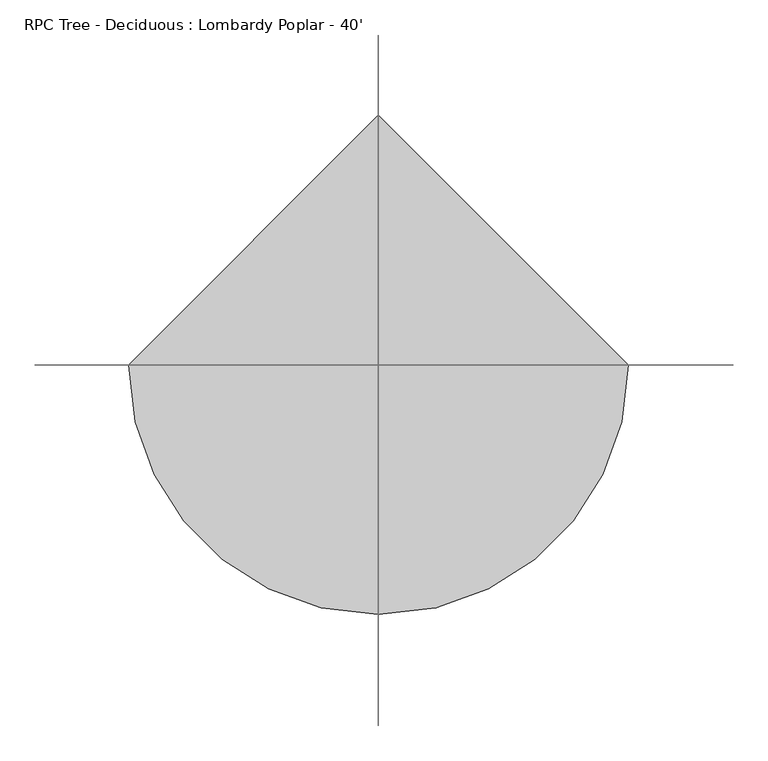
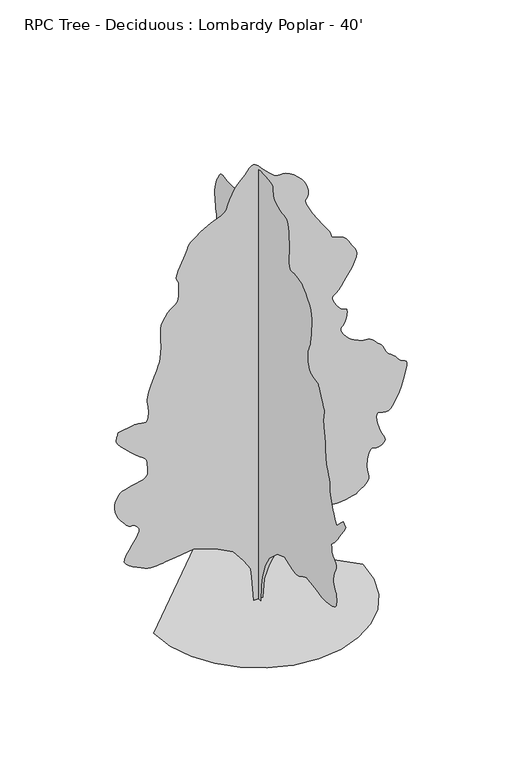
"""IFC4 building model written with IfcOpenShell, lengths in millimetres: geographic element geometry, RPC Tree - Deciduous : Lombardy Poplar - 40'."""

from ifc_helpers import new_model, si_unit, origin, place, context, project, spatial, triangles, source, transform, mapped, element, save


def rpc_tree_deciduous_lombardy_poplar_40_01077960(model_context):
    return source(origin(), model_context, "Body", "Tessellation", [
        triangles([(0.0009695, 113.8156909, 0.0), (0.0009695, -104.8345258, 0.0), (0.0009695, -123.055434, 437.3009239), (0.0009695, -177.7179314, 728.8340738), (0.0009695, -323.483707, 1129.6911467), (0.0009695, -505.6928613, 1439.4461494), (0.0009695, -870.1086628, 1767.420607), (0.0009695, -1216.3049732, 1894.9664555), (0.0009695, -1398.5142002, 1822.0838402), (0.0009695, -1476.390406, 1795.1523445), (0.0009695, -1552.9941605, 1770.6083485), (0.0009695, -1627.0451637, 1750.8472), (0.0009695, -1697.2735806, 1738.2588696), (0.0009695, -1762.3991112, 1735.2286766), (0.0009695, -1821.1516296, 1744.1542946), (0.0009695, -1872.2563591, 1767.420607), (0.0009695, -1919.1091679, 1797.0624023), (0.0009695, -1965.9644474, 1823.8364948), (0.0009695, -2012.8172562, 1848.2204716), (0.0009695, -2059.6700649, 1870.6891582), (0.0009695, -2106.5227283, 1891.7279903), (0.0009695, -2153.3780079, 1911.8067066), (0.0009695, -2200.2308167, 1931.4103065), (0.0009695, -2582.8711235, 1876.7470734), (0.0009695, -2649.2156204, 1861.2353748), (0.0009695, -2715.4080917, 1846.3611374), (0.0009695, -2781.27006, 1832.7619675), (0.0009695, -2846.6750793, 1821.0754715), (0.0009695, -2911.4196739, 1811.9366398), (0.0009695, -2975.3765259, 1805.987875), (0.0009695, -3038.3939003, 1803.8619873), (0.0009695, -3111.6472778, 1806.252103), (0.0009695, -3200.5217949, 1814.0625275), (0.0009695, -3296.0764275, 1828.2459641), (0.0009695, -3389.4213112, 1849.7596218), (0.0009695, -3471.5901329, 1879.5614365), (0.0009695, -3533.6930283, 1918.6062916), (0.0009695, -3566.7892639, 1967.8516869), (0.0009695, -3579.2353065, 2021.4507408), (0.0009695, -3585.9154221, 2073.1371208), (0.0009695, -3587.8205383, 2123.2333363), (0.0009695, -3585.9154221, 2172.0521587), (0.0009695, -3581.1401321, 2219.915807), (0.0009695, -3574.4347275, 2267.139378), (0.0009695, -3566.7892639, 2314.0455265), (0.0009695, -3532.0422569, 2353.5170998), (0.0009695, -3499.7078934, 2395.5361919), (0.0009695, -3472.1235306, 2442.6555542), (0.0009695, -3451.7273918, 2497.4231415), (0.0009695, -3440.907122, 2562.3988266), (0.0009695, -3441.9992065, 2640.0972816), (0.0009695, -3457.4677391, 2733.1372421), (0.0009695, -3484.5187042, 2825.1865654), (0.0009695, -3515.3799019, 2900.6752716), (0.0009695, -3544.9708282, 2963.0830902), (0.0009695, -3568.1862717, 3015.940329), (0.0009695, -3579.9210205, 3062.7525879), (0.0009695, -3575.0695724, 3106.9993057), (0.0009695, -3548.5775848, 3152.2110809), (0.0009695, -3509.7918709, 3193.1050964), (0.0009695, -3472.6063499, 3225.0836678), (0.0009695, -3438.6212151, 3252.6171616), (0.0009695, -3409.3857903, 3280.1253662), (0.0009695, -3386.5511375, 3312.1039375), (0.0009695, -3371.6668716, 3352.997953), (0.0009695, -3366.3581841, 3407.3030685), (0.0009695, -3362.7005585, 3460.5158089), (0.0009695, -3354.9027786, 3498.4634926), (0.0009695, -3347.7145546, 3525.8699593), (0.0009695, -3345.9620453, 3547.5360786), (0.0009695, -3354.4202499, 3568.2624298), (0.0009695, -3377.8388786, 3592.7987228), (0.0009695, -3421.0188011, 3625.9458275), (0.0009695, -3481.5215034, 3679.8698616), (0.0009695, -3552.5654228, 3760.5655174), (0.0009695, -3632.3465996, 3863.5624283), (0.0009695, -3719.1381042, 3984.4155167), (0.0009695, -3811.2130074, 4118.6541252), (0.0009695, -3906.7676399, 4261.8084686), (0.0009695, -4004.1003616, 4409.432888), (0.0009695, -3894.7788368, 4518.779702), (0.0009695, -3749.0086647, 4391.221209), (0.0009695, -3603.2382019, 4227.2390671), (0.0009695, -3579.7434151, 4258.785688), (0.0009695, -3555.9689941, 4292.2630051), (0.0009695, -3531.5088593, 4329.5499733), (0.0009695, -3506.1342453, 4372.5775795), (0.0009695, -3479.4643616, 4423.2506493), (0.0009695, -3451.1939941, 4483.4992973), (0.0009695, -3421.0188011, 4555.2033508), (0.0009695, -3390.0055779, 4628.5837555), (0.0009695, -3360.2623352, 4695.8683113), (0.0009695, -3333.0587631, 4762.2383881), (0.0009695, -3309.6910034, 4832.7233299), (0.0009695, -3291.4028755, 4912.4536377), (0.0009695, -3279.5158104, 5006.5351044), (0.0009695, -3275.248629, 5120.0473618), (0.0009695, -3267.0697678, 5234.8554703), (0.0009695, -3245.5050957, 5333.3820145), (0.0009695, -3215.0252701, 5421.7481323), (0.0009695, -3180.0747871, 5505.9238083), (0.0009695, -3145.0993057, 5592.0551788), (0.0009695, -3114.6191895, 5686.1110657), (0.0009695, -3093.0545174, 5794.238768), (0.0009695, -3079.5672592, 5892.1298859), (0.0009695, -3069.8899429, 5959.4403122), (0.0009695, -3063.4130127, 6007.9286316), (0.0009695, -3059.4760437, 6049.4319122), (0.0009695, -3057.4691895, 6095.6854843), (0.0009695, -3056.7073174, 6158.5246719), (0.0009695, -3056.6055794, 6249.735965), (0.0009695, -3052.5671631, 6343.1320084), (0.0009695, -3042.1532639, 6412.2958099), (0.0009695, -3027.9291321, 6468.709227), (0.0009695, -3012.4097305, 6523.8523727), (0.0009695, -2998.1858894, 6589.2065231), (0.0009695, -2987.7716995, 6676.2017944), (0.0009695, -2983.7332832, 6796.3688782), (0.0009695, -2989.2957344, 6908.7381821), (0.0009695, -3001.5638809, 6976.78461), (0.0009695, -3013.8576073, 7018.6948425), (0.0009695, -3019.4200584, 7052.6288177), (0.0009695, -3011.6222786, 7096.7737976), (0.0009695, -2983.7332832, 7169.2908829), (0.0009695, -2929.0723755, 7288.340593), (0.0009695, -2866.7410057, 7418.1088348), (0.0009695, -2818.7857933, 7514.4256302), (0.0009695, -2782.7688057, 7582.8528488), (0.0009695, -2756.3021072, 7628.9541046), (0.0009695, -2737.0233421, 7658.3418457), (0.0009695, -2722.5201576, 7676.5535248), (0.0009695, -2710.4043274, 7689.2027527), (0.0009695, -2636.5666832, 7701.2421341), (0.0009695, -2564.8117607, 7715.3901077), (0.0009695, -2497.1818771, 7733.6523651), (0.0009695, -2435.7748695, 7758.1380798), (0.0009695, -2382.6507866, 7790.9296829), (0.0009695, -2339.8900246, 7834.0584457), (0.0009695, -2309.5548122, 7889.6335419), (0.0009695, -2289.3160767, 7951.0257248), (0.0009695, -2274.8152176, 8010.5377899), (0.0009695, -2265.0921192, 8068.4243729), (0.0009695, -2259.1968395, 8125.0662643), (0.0009695, -2256.1691174, 8180.7425171), (0.0009695, -2255.0515984, 8235.7589264), (0.0009695, -2254.8940498, 8290.4707031), (0.0009695, -2285.970932, 8345.7405853), (0.0009695, -2316.0901691, 8404.491069), (0.0009695, -2344.2968777, 8470.25159), (0.0009695, -2369.6358833, 8546.5277481), (0.0009695, -2391.1521572, 8636.8495605), (0.0009695, -2407.8857288, 8744.6726303), (0.0009695, -2418.8812786, 8873.551973), (0.0009695, -2430.0903328, 9004.9206985), (0.0009695, -2443.8493767, 9121.3031296), (0.0009695, -2453.7833633, 9227.8303482), (0.0009695, -2453.5168098, 9329.5572784), (0.0009695, -2436.6765587, 9431.5888412), (0.0009695, -2396.8874176, 9539.0561188), (0.0009695, -2327.7766651, 9657.0390335), (0.0009695, -2247.8811058, 9768.2398041), (0.0009695, -2177.228587, 9854.8798645), (0.0009695, -2111.6764835, 9921.4269653), (0.0009695, -2047.0792637, 9972.3796692), (0.0009695, -1979.2969185, 10012.156311), (0.0009695, -1904.1815907, 10045.2519653), (0.0009695, -1817.5931259, 10076.1128723), (0.0009695, -1725.5334835, 10094.8326599), (0.0009695, -1638.891679, 10096.3058258), (0.0009695, -1560.8554539, 10092.3688568), (0.0009695, -1494.6124043, 10094.8326599), (0.0009695, -1443.3501263, 10115.4325653), (0.0009695, -1410.2540359, 10166.0038971), (0.0009695, -1398.5142002, 10258.3319824), (0.0009695, -1400.4267288, 10362.6756134), (0.0009695, -1404.8895378, 10448.1971375), (0.0009695, -1409.9898079, 10525.1087219), (0.0009695, -1413.8125397, 10603.619046), (0.0009695, -1414.4501461, 10693.9414398), (0.0009695, -1409.9898079, 10806.2345856), (0.0009695, -1398.5142002, 10950.7350677), (0.0009695, -1382.6849339, 11097.4458801), (0.0009695, -1365.5779839, 11211.9737732), (0.0009695, -1345.9235149, 11297.8255096), (0.0009695, -1322.4438435, 11358.4811096), (0.0009695, -1293.8637566, 11397.4694275), (0.0009695, -1258.9083321, 11418.297226), (0.0009695, -1216.3049732, 11424.470105), (0.0009695, -1155.4822323, 11429.9813965), (0.0009695, -1073.3006933, 11446.3641174), (0.0009695, -979.6484882, 11473.2380585), (0.0009695, -884.3986336, 11510.3218414), (0.0009695, -797.4393339, 11557.2608368), (0.0009695, -728.6460766, 11613.8015717), (0.0009695, -687.9020519, 11679.5615112), (0.0009695, -672.8677952, 11749.3607391), (0.0009695, -668.0341513, 11816.289212), (0.0009695, -663.5180752, 11877.4785004), (0.0009695, -649.4413908, 11930.0811035), (0.0009695, -615.9210531, 11971.2041748), (0.0009695, -553.0790314, 11997.9757965), (0.0009695, -451.0296281, 12007.5263763), (0.0009695, -327.7864603, 12011.2087097), (0.0009695, -210.2816959, 12019.0070709), (0.0009695, -102.0189364, 12026.1694244), (0.0009695, -6.5056406, 12027.9216431), (0.0009695, 72.7523407, 12019.4895996), (0.0009695, 132.2489498, 11996.0700989), (0.0009695, 168.4781792, 11952.8657593), (0.0009695, 190.2581361, 11903.7920105), (0.0009695, 211.0820467, 11861.400412), (0.0009695, 234.4553475, 11819.0076508), (0.0009695, 263.8852554, 11769.9094849), (0.0009695, 302.8767344, 11707.4505066), (0.0009695, 354.9364746, 11624.9008942), (0.0009695, 423.5697126, 11515.57966), (0.0009695, 499.5867296, 11399.1204895), (0.0009695, 572.09851, 11297.9778259), (0.0009695, 642.0601553, 11209.5867096), (0.0009695, 710.4292379, 11131.3798553), (0.0009695, 778.1582434, 11060.8446259), (0.0009695, 846.2072874, 10995.3881561), (0.0009695, 915.531399, 10932.4978088), (0.0009695, 983.7404623, 10880.5556305), (0.0009695, 1048.444289, 10847.0786041), (0.0009695, 1110.5954372, 10828.282077), (0.0009695, 1171.1565662, 10820.3069824), (0.0009695, 1231.077618, 10819.3407623), (0.0009695, 1291.3160923, 10821.5766724), (0.0009695, 1352.8322502, 10823.1765747), (0.0009695, 1419.1287849, 10828.7646057), (0.0009695, 1490.5254444, 10841.0324615), (0.0009695, 1563.194846, 10853.3014801), (0.0009695, 1633.3164379, 10858.8639313), (0.0009695, 1697.0626923, 10851.0655701), (0.0009695, 1750.6084064, 10823.1765747), (0.0009695, 1790.1333195, 10768.5159576), (0.0009695, 1824.1844387, 10700.9526398), (0.0009695, 1861.7408672, 10636.2333344), (0.0009695, 1899.617189, 10570.5745514), (0.0009695, 1934.6234825, 10500.1404785), (0.0009695, 1963.5743317, 10421.0953033), (0.0009695, 1983.2847565, 10329.6299561), (0.0009695, 1990.5617832, 10221.8830444), (0.0009695, 1988.4357502, 10111.0130676), (0.0009695, 1982.4871307, 10010.9877777), (0.0009695, 1973.3507698, 9919.2433777), (0.0009695, 1961.6642738, 9833.2381622), (0.0009695, 1948.0651039, 9750.4350769), (0.0009695, 1933.1908665, 9668.2656738), (0.0009695, 1917.6791679, 9584.1667374), (0.0009695, 1914.3314072, 9505.3761978), (0.0009695, 1931.0649788, 9438.0663528), (0.0009695, 1961.1842159, 9378.0967575), (0.0009695, 1997.9989746, 9321.3025497), (0.0009695, 2034.813588, 9263.5682831), (0.0009695, 2064.9328251, 9200.7290955), (0.0009695, 2081.6663967, 9128.6439606), (0.0009695, 2081.1888096, 9058.6668365), (0.0009695, 2066.6854797, 9001.7964706), (0.0009695, 2041.9840805, 8953.1808334), (0.0009695, 2010.9071983, 8908.0707962), (0.0009695, 1977.2826519, 8861.6904877), (0.0009695, 1944.9307022, 8809.2646179), (0.0009695, 1917.6791679, 8745.9934799), (0.0009695, 1901.8472855, 8673.7048691), (0.0009695, 1900.361475, 8598.2164536), (0.0009695, 1911.9412914, 8520.8229218), (0.0009695, 1935.3142834, 8442.7939636), (0.0009695, 1969.2055286, 8365.374852), (0.0009695, 2012.3422852, 8289.8864365), (0.0009695, 2063.4443985, 8217.5978256), (0.0009695, 2116.1951031, 8158.060762), (0.0009695, 2166.3955273, 8113.7884644), (0.0009695, 2215.9584904, 8075.6123062), (0.0009695, 2266.796521, 8034.2101822), (0.0009695, 2320.8222931, 7980.4134659), (0.0009695, 2379.9457191, 7904.924469), (0.0009695, 2446.0820892, 7798.5239868), (0.0009695, 2515.4595406, 7684.1478287), (0.0009695, 2583.8870499, 7588.5931961), (0.0009695, 2652.6194824, 7508.3039108), (0.0009695, 2722.9518173, 7439.8511124), (0.0009695, 2796.1546165, 7379.653624), (0.0009695, 2873.4972794, 7324.2558426), (0.0009695, 2956.2759476, 7270.103334), (0.0009695, 3039.9940933, 7227.3042023), (0.0009695, 3119.5720848, 7202.0063278), (0.0009695, 3195.3148453, 7185.0137604), (0.0009695, 3267.5522964, 7167.0555542), (0.0009695, 3336.6149414, 7138.9125046), (0.0009695, 3402.807122, 7091.3130844), (0.0009695, 3466.4593414, 7015.0113464), (0.0009695, 3525.2604034, 6921.5903046), (0.0009695, 3575.4506538, 6829.7441666), (0.0009695, 3615.1508469, 6741.0728348), (0.0009695, 3642.3797081, 6657.2023727), (0.0009695, 3655.3082794, 6579.6815231), (0.0009695, 3651.9552864, 6510.1619293), (0.0009695, 3630.4414833, 6450.1673355), (0.0009695, 3590.004998, 6392.5348068), (0.0009695, 3534.6075073, 6330.4316208), (0.0009695, 3469.3295151, 6266.1192673), (0.0009695, 3399.2512344, 6201.7813339), (0.0009695, 3329.5028755, 6139.6781479), (0.0009695, 3265.1646515, 6082.0456192), (0.0009695, 3211.3676445, 6031.0934967), (0.0009695, 3161.7869499, 5985.0939789), (0.0009695, 3109.3613708, 5939.7298874), (0.0009695, 3057.8758507, 5893.4001572), (0.0009695, 3011.1906189, 5844.5304657), (0.0009695, 2973.1159081, 5791.5209106), (0.0009695, 2947.4366615, 5732.7710083), (0.0009695, 2938.0386887, 5666.680275), (0.0009695, 2934.1778778, 5597.4141541), (0.0009695, 2924.8816429, 5529.7235184), (0.0009695, 2913.6547119, 5463.0235199), (0.0009695, 2904.0535538, 5396.6025742), (0.0009695, 2899.5323181, 5329.8764145), (0.0009695, 2903.6218941, 5262.2113586), (0.0009695, 2919.8270096, 5192.9452377), (0.0009695, 2944.8458313, 5126.3719757), (0.0009695, 2972.7351173, 5066.5046997), (0.0009695, 3003.0117577, 5012.2248734), (0.0009695, 3035.1935143, 4962.3901245), (0.0009695, 3068.8231476, 4915.908078), (0.0009695, 3103.4178383, 4871.6613602), (0.0009695, 3138.4697685, 4828.5323067), (0.0009695, 3181.1415825, 4835.3141602), (0.0009695, 3222.035598, 4836.0760323), (0.0009695, 3259.4243042, 4824.696785), (0.0009695, 3291.5807716, 4795.1567276), (0.0009695, 3316.7013313, 4741.4102989), (0.0009695, 3333.0587631, 4657.3619408), (0.0009695, 3338.9008484, 4536.9916718), (0.0009695, 3338.9008484, 3935.6984322), (0.0009695, 3345.6065437, 3757.6444748), (0.0009695, 3361.2273926, 3611.1377197), (0.0009695, 3379.0582809, 3492.0371407), (0.0009695, 3392.4440918, 3396.2031647), (0.0009695, 3394.6791298, 3319.4953468), (0.0009695, 3379.0582809, 3257.747953), (0.0009695, 3338.9008484, 3206.8719887), (0.0009695, 3281.573243, 3178.2461197), (0.0009695, 3221.7053856, 3174.1568344), (0.0009695, 3163.4380119, 3176.747374), (0.0009695, 3110.9106949, 3168.187722), (0.0009695, 3068.2388809, 3130.6466995), (0.0009695, 3039.6130119, 3046.21726), (0.0009695, 3029.1482437, 2897.119384), (0.0009695, 3036.0571243, 2732.8070297), (0.0009695, 3053.1514297, 2608.9823204), (0.0009695, 3075.0460236, 2517.0268867), (0.0009695, 3096.3057724, 2448.3400909), (0.0009695, 3111.4949615, 2394.3144642), (0.0009695, 3115.2034561, 2346.3441364), (0.0009695, 3102.0208305, 2295.8261444), (0.0009695, 3089.0669701, 2254.1778145), (0.0009695, 3089.803553, 2232.6106716), (0.0009695, 3093.4355988, 2222.1992432), (0.0009695, 3089.0669701, 2214.0179111), (0.0009695, 3065.9021049, 2199.1436737), (0.0009695, 3013.0954445, 2168.6510582), (0.0009695, 2919.8270096, 2113.6169174), (0.0009695, 2822.3419716, 2052.8450455), (0.0009695, 2753.55867, 2008.9666191), (0.0009695, 2697.5010452, 1978.7940422), (0.0009695, 2638.2683235, 1959.1395733), (0.0009695, 2559.9350235, 1946.8154709), (0.0009695, 2446.5088074, 1938.6341389), (0.0009695, 2282.0948605, 1931.4103065), (0.0009695, 2105.8903542, 1933.6938881), (0.0009695, 1963.4702682, 1951.9132702), (0.0009695, 1848.4591198, 1979.6982021), (0.0009695, 1754.4869488, 2010.665934), (0.0009695, 1675.1755108, 2038.4483952), (0.0009695, 1604.1522297, 2056.670248), (0.0009695, 1535.0414772, 2058.9536842), (0.0009695, 1460.510416, 2049.0198429), (0.0009695, 1378.3312752, 2035.2631245), (0.0009695, 1289.7769421, 2018.3163391), (0.0009695, 1196.1221935, 1998.8218895), (0.0009695, 1098.6447859, 1977.4122952), (0.0009695, 998.6146271, 1954.7301041), (0.0009695, 897.3120169, 1931.4103065), (0.0009695, 532.8936719, 1639.8747585), (0.0009695, 314.2457534, 1166.1349977), (0.0009695, 168.4781792, 601.2881527), (120.1776209, 0.0005334, 0.0085345), (-116.69275, 0.0005334, 0.0085345), (-171.3552383, 0.0004849, 655.9590162), (-207.7973272, 0.0004849, 911.0508585), (-390.006209, 0.0004607, 1202.5839357), (-663.3174334, 0.0004364, 1548.7803188), (-1137.0596649, 0.0004122, 1803.8721611), (-1720.1284355, 0.0004122, 1986.078772), (-2193.8681236, 0.0004122, 1931.4180096), (-2467.1819641, 0.0004122, 1894.9766293), (-2533.7959213, 0.0004122, 1885.46689), (-2607.4327057, 0.0004122, 1874.6820831), (-2686.1473778, 0.0004122, 1865.812421), (-2768.0621452, 0.0004122, 1862.0405582), (-2851.2468933, 0.0004122, 1866.556707), (-2933.7967964, 0.0004122, 1882.5459927), (-3013.8067383, 0.0004122, 1913.1960114), (-3104.2814484, 0.0004122, 1955.5886272), (-3210.9865631, 0.0004122, 2004.6715324), (-3321.222567, 0.0004122, 2060.4522846), (-3422.2126236, 0.0004122, 2122.9234715), (-3501.2066391, 0.0003879, 2192.0875637), (-3545.4533569, 0.0003879, 2267.9445614), (-3542.2021019, 0.0003879, 2350.4969353), (-3495.1869484, 0.0003879, 2447.2326004), (-3424.930481, 0.0003879, 2559.9094437), (-3343.8031654, 0.0003637, 2679.898922), (-3264.2757523, 0.0003637, 2798.6437088), (-3198.7692856, 0.0003637, 2907.4824142), (-3159.7295174, 0.0003394, 2997.8300972), (-3159.5772011, 0.0003394, 3061.1015259), (-3182.9958298, 0.0003394, 3103.1893639), (-3206.4147491, 0.0003394, 3136.6411011), (-3229.8589577, 0.0003394, 3162.9554832), (-3253.2775864, 0.0003394, 3183.5039383), (-3276.6962151, 0.0003394, 3199.7599228), (-3300.1404236, 0.0003394, 3213.1457336), (-3323.559343, 0.0003394, 3225.1089569), (-3347.1558678, 0.0003394, 3221.5783585), (-3371.6921608, 0.0003394, 3220.486274), (-3398.1335701, 0.0003394, 3224.1438995), (-3427.4704422, 0.0003394, 3234.9897491), (-3460.6175468, 0.0003394, 3255.3858879), (-3498.5396507, 0.0003394, 3287.7199608), (-3542.2021019, 0.0003394, 3334.4304817), (-3593.6370438, 0.0003394, 3395.5174507), (-3650.1519081, 0.0003152, 3468.3897469), (-3705.7270042, 0.0003152, 3551.4730476), (-3754.2664833, 0.0003152, 3643.1668694), (-3789.7500732, 0.0003152, 3741.8713097), (-3806.1330849, 0.0002909, 3845.9855942), (-3797.2937988, 0.0002909, 3953.9354004), (-3771.4366562, 0.0002909, 4051.5730453), (-3739.8138771, 0.0002909, 4128.1791252), (-3701.2057686, 0.0002909, 4187.2342415), (-3654.2920624, 0.0002667, 4232.2937004), (-3597.828067, 0.0002667, 4266.812233), (-3530.518222, 0.0002667, 4294.3457268), (-3451.117836, 0.0002667, 4318.3486221), (-3356.8078949, 0.0002667, 4338.3131012), (-3252.3378181, 0.0002667, 4355.4326958), (-3147.5122398, 0.0002667, 4375.7270966), (-3052.2622398, 0.0002667, 4405.2674446), (-2976.4689011, 0.0002667, 4450.0981384), (-2929.9868546, 0.0002667, 4516.2906097), (-2922.6971832, 0.0002667, 4609.8895477), (-2933.5936111, 0.0002425, 4707.6283493), (-2938.4197701, 0.0002425, 4784.9713028), (-2942.3058701, 0.0002425, 4846.0582718), (-2950.332415, 0.0002425, 4895.0291199), (-2967.578746, 0.0002425, 4936.0504532), (-2999.2018158, 0.0002425, 4973.2359741), (-3050.2556763, 0.0002425, 5010.7517075), (-3135.4978569, 0.0002182, 5072.041571), (-3254.8777794, 0.0002182, 5168.7141586), (-3391.1232422, 0.0002182, 5287.0778641), (-3527.0637817, 0.0002182, 5413.3916656), (-3645.4783562, 0.000194, 5533.9906998), (-3729.1459236, 0.000194, 5635.1333633), (-3760.8704407, 0.000194, 5703.129213), (-3759.2702477, 0.000194, 5747.3247711), (-3754.799881, 0.000194, 5786.7456207), (-3747.9418694, 0.000194, 5822.178923), (-3739.1787415, 0.0001697, 5854.4112579), (-3728.9933167, 0.0001697, 5884.2815277), (-3717.8428345, 0.0001697, 5912.5263153), (-3706.2095329, 0.0001697, 5940.0089401), (-3268.8984352, 0.0001697, 6012.8818176), (-3174.1312546, 0.0001697, 6014.48172), (-3093.0545174, 0.0001697, 5998.8605804), (-3026.0240158, 0.0001697, 5982.2743835), (-2973.319384, 0.0001697, 5981.0046936), (-2935.2955421, 0.0001697, 6011.2813339), (-2912.232415, 0.0001697, 6089.3864502), (-2904.4852135, 0.0001697, 6231.5242859), (-2910.9624344, 0.0001455, 6377.1421417), (-2925.0848282, 0.0001455, 6470.4870255), (-2938.9022987, 0.0001455, 6535.1301727), (-2944.4394608, 0.0001455, 6594.6678177), (-2933.6953491, 0.0001212, 6672.7217743), (-2898.7448662, 0.0001212, 6792.8126999), (-2831.5873375, 0.0001212, 6978.5879883), (-2754.346122, 9.7e-05, 7175.5649185), (-2693.3861801, 9.7e-05, 7325.0435852), (-2647.0567406, 9.7e-05, 7444.2456116), (-2613.8081886, 7.27e-05, 7550.3920395), (-2592.0150421, 7.27e-05, 7660.678331), (-2580.127977, 7.27e-05, 7792.3011108), (-2576.4956406, 4.85e-05, 7962.5064194), (-2580.0009499, 4.85e-05, 8135.9626923), (-2586.7063545, 4.85e-05, 8272.4363388), (-2590.8467995, 2.42e-05, 8381.8087326), (-2586.7063545, 2.42e-05, 8473.985083), (-2568.5455444, 2.42e-05, 8558.8211838), (-2530.6106506, 2.42e-05, 8646.1972458), (-2467.1819641, 0.0, 8746.0190598), (-2393.5550629, 0.0, 8838.8046753), (-2328.8511635, 0.0, 8903.8797729), (-2273.0728821, 0.0, 8949.1932861), (-2226.2200733, 0.0, 8982.7208908), (-2188.2902664, 0.0, 9012.4138458), (-2159.2860775, 0.0, 9046.2460831), (-2139.2048904, 0.0, 9092.1950226), (-2125.7124001, -2.42e-05, 9135.3493652), (-2116.0452576, -2.42e-05, 9162.8575699), (-2109.5630951, -2.42e-05, 9185.920697), (-2105.6338291, -2.42e-05, 9215.6642303), (-2103.6144756, -2.42e-05, 9263.2636505), (-2102.8701897, -2.42e-05, 9339.8700211), (-2102.7661263, -2.42e-05, 9456.6332428), (-2113.0708752, -4.85e-05, 9567.5549606), (-2136.1264446, -4.85e-05, 9634.4840149), (-2160.137043, -4.85e-05, 9680.3817947), (-2173.3094948, -4.85e-05, 9728.1846909), (-2163.855566, -4.85e-05, 9800.8540924), (-2119.9745235, -7.27e-05, 9921.3258087), (-2029.8808949, -7.27e-05, 10112.5618103), (-1939.4672276, -7.27e-05, 10305.830246), (-1888.8958958, -9.7e-05, 10431.5097839), (-1857.7656738, -9.7e-05, 10511.3165405), (-1825.6805683, -9.7e-05, 10566.8654755), (-1772.2389175, -9.7e-05, 10619.9006104), (-1677.0450188, -9.7e-05, 10692.0369049), (-1519.6973557, -0.0001212, 10804.9648956), (-1341.6868549, -0.0001212, 10917.309201), (-1195.5481733, -0.0001212, 10985.3806274), (-1077.4586517, -0.0001212, 11027.29086), (-983.5905441, -0.0001212, 11061.2248352), (-910.1237349, -0.0001212, 11105.3698151), (-853.2303326, -0.0001455, 11177.8874817), (-809.0852074, -0.0001455, 11296.9371918), (-759.9464916, -0.0001455, 11440.4714539), (-694.8717573, -0.0001697, 11572.8563965), (-620.2365601, -0.0001697, 11691.8293671), (-542.413585, -0.0001697, 11795.2079407), (-467.775808, -0.0001697, 11880.7294647), (-402.7036534, -0.0001697, 11946.1847717), (-353.5649014, -0.000194, 11989.3146973), (-315.2642959, -0.000194, 12029.8529205), (-276.9611651, -0.000194, 12081.541626), (-236.4299363, -0.000194, 12133.2303314), (-191.4351718, -0.000194, 12173.7685547), (-139.7475292, -0.000194, 12191.9802338), (-79.1353495, -0.000194, 12176.7404663), (-7.3676139, -0.000194, 12116.8731903), (68.4904824, -0.000194, 12035.3130524), (139.8862108, -0.000194, 11962.0605469), (206.8199341, -0.0001697, 11896.4517609), (269.290376, -0.0001697, 11837.8797546), (327.3013518, -0.0001697, 11785.6573608), (380.8469934, -0.0001697, 11739.1753143), (429.9324057, -0.0001697, 11697.7987701), (477.3160323, -0.0001697, 11672.4491547), (527.8899076, -0.0001697, 11666.8622864), (584.8366133, -0.0001697, 11669.5795624), (651.343891, -0.0001697, 11669.0970337), (730.6019165, -0.0001697, 11653.9584229), (825.7958879, -0.0001697, 11612.684198), (940.1160175, -0.0001455, 11533.7913391), (1053.1051964, -0.0001455, 11434.3508972), (1143.4680674, -0.0001455, 11338.4148926), (1213.1096741, -0.0001455, 11245.0194305), (1263.9477047, -0.0001455, 11153.2238708), (1297.8921444, -0.0001212, 11062.0631561), (1316.8558125, -0.0001212, 10970.5978088), (1322.7537083, -0.0001212, 10877.8371918), (1310.6404942, -0.0001212, 10807.3019623), (1283.8688725, -0.0001212, 10768.6426941), (1256.7747414, -0.0001212, 10740.1444336), (1243.7064983, -9.7e-05, 10700.2154755), (1259.0074539, -9.7e-05, 10627.1141235), (1317.0158318, -9.7e-05, 10499.1998383), (1432.0777039, -7.27e-05, 10294.7809204), (1568.3356659, -7.27e-05, 10074.4362305), (1681.0074223, -4.85e-05, 9906.365094), (1771.0503273, -4.85e-05, 9780.3565063), (1839.4167938, -4.85e-05, 9686.22388), (1887.067083, -4.85e-05, 9613.757373), (1914.9562237, -4.85e-05, 9552.772142), (1924.041861, -2.42e-05, 9493.0571823), (1943.5896503, -2.42e-05, 9444.2892288), (1995.6494087, -2.42e-05, 9415.2822784), (2070.3380184, -2.42e-05, 9394.5812164), (2157.7773033, -2.42e-05, 9370.6797684), (2248.0842911, -2.42e-05, 9332.0972397), (2331.3809509, -2.42e-05, 9267.4035141), (2397.7841652, -2.42e-05, 9165.0928986), (2454.6240097, 0.0, 9055.2379761), (2511.1467224, 0.0, 8968.9542892), (2560.341394, 0.0, 8896.3866257), (2595.190139, 0.0, 8827.6541931), (2608.6773972, 0.0, 8752.8512009), (2593.7931313, 2.42e-05, 8662.1230179), (2543.5520119, 2.42e-05, 8545.5876892), (2481.3447624, 2.42e-05, 8432.1260101), (2431.8886242, 2.42e-05, 8349.5508179), (2390.080275, 2.42e-05, 8286.457576), (2350.8220608, 4.85e-05, 8231.3138489), (2309.0163277, 4.85e-05, 8172.6656845), (2259.5600441, 4.85e-05, 8099.0312256), (2197.3530853, 4.85e-05, 7998.9553574), (2127.0206051, 4.85e-05, 7904.0355698), (2060.8307499, 7.27e-05, 7844.1677124), (2005.159148, 7.27e-05, 7805.3311295), (1966.378521, 7.27e-05, 7773.5051651), (1950.8666771, 7.27e-05, 7734.6685822), (1964.9992447, 7.27e-05, 7674.8007248), (2015.1464745, 7.27e-05, 7579.8815186), (2080.6452381, 7.27e-05, 7478.1545883), (2137.5387131, 9.7e-05, 7404.1387573), (2187.2590794, 9.7e-05, 7353.262793), (2231.2468014, 9.7e-05, 7320.852562), (2270.9265015, 9.7e-05, 7302.3106705), (2307.7412601, 9.7e-05, 7293.0141449), (2343.1207867, 9.7e-05, 7288.340593), (2346.839455, 9.7e-05, 7260.6544922), (2349.4429298, 9.7e-05, 7230.9109589), (2349.8136921, 9.7e-05, 7197.027562), (2346.839455, 9.7e-05, 7156.9212891), (2339.4022636, 9.7e-05, 7108.5341263), (2326.3873604, 0.0001212, 7049.7842239), (2306.6795517, 0.0001212, 6978.5879883), (2277.832766, 0.0001212, 6914.427951), (2243.2507198, 0.0001212, 6871.273027), (2210.5813477, 0.0001212, 6838.9901138), (2187.4724384, 0.0001212, 6807.3158844), (2181.5771587, 0.0001212, 6766.0922379), (2200.5406815, 0.0001212, 6705.1064255), (2252.0163185, 0.0001455, 6614.1747665), (2322.1379105, 0.0001455, 6519.5090332), (2391.3020027, 0.0001455, 6450.3452316), (2458.553421, 0.0001455, 6400.9424332), (2522.9372818, 0.0001455, 6365.5602905), (2583.5059685, 0.0001455, 6338.4584564), (2639.2842499, 0.0001455, 6313.9221634), (2689.322184, 0.0001455, 6286.184903), (2738.2427444, 0.0001455, 6263.7822006), (2790.6680328, 0.0001455, 6254.1048843), (2845.659153, 0.0001697, 6249.8632828), (2902.2248863, 0.0001697, 6243.6909851), (2959.4507538, 0.0001697, 6228.2989014), (3016.3466995, 0.0001697, 6196.3200394), (3071.9473755, 0.0001697, 6140.4403107), (3121.4519119, 0.0001697, 6084.0774719), (3162.3712166, 0.0001697, 6048.746489), (3197.2199615, 0.0001697, 6024.2607742), (3228.5633972, 0.0001697, 6000.4104858), (3258.9417755, 0.0001697, 5966.9840378), (3290.9203468, 0.0001697, 5913.8215851), (3327.0390724, 0.000194, 5830.687706), (3367.3235321, 0.000194, 5746.3091354), (3410.4525856, 0.000194, 5689.0573975), (3457.0869484, 0.000194, 5648.0366455), (3507.8614655, 0.000194, 5612.4510269), (3563.4365616, 0.000194, 5571.430275), (3624.4217926, 0.000194, 5514.178537), (3691.4522942, 0.0002182, 5429.8255463), (3759.9306725, 0.0002182, 5354.920816), (3822.0335678, 0.0002182, 5319.208461), (3873.620826, 0.0002182, 5301.6827866), (3910.5270035, 0.0002182, 5281.2863571), (3928.6625244, 0.0002182, 5236.989061), (3923.8110764, 0.0002182, 5147.7334625), (3891.883374, 0.0002425, 4992.5144485), (3839.8897453, 0.0002425, 4801.4304726), (3779.2600159, 0.0002667, 4621.8274818), (3712.6105957, 0.0002667, 4458.4801849), (3642.4302864, 0.0002667, 4316.1641624), (3571.3104996, 0.0002909, 4199.6799934), (3501.7653259, 0.0002909, 4113.777388), (3436.3605972, 0.0002909, 4063.2569252), (3368.5935127, 0.0002909, 4052.055574), (3295.6956367, 0.0002909, 4067.2956322), (3225.9981468, 0.0002909, 4088.6059593), (3167.7813515, 0.0002909, 4095.5657089), (3129.3258499, 0.0002909, 4067.7781609), (3118.9119507, 0.0002909, 3984.8471764), (3144.8452515, 0.0002909, 3826.3769073), (3196.8388802, 0.0003152, 3648.5264259), (3252.998243, 0.0003152, 3514.6686081), (3304.0521034, 0.0003152, 3415.2278755), (3340.7550957, 0.0003394, 3340.6280685), (3353.8615631, 0.0003394, 3281.3444778), (3334.1764275, 0.0003394, 3227.8015251), (3272.3784554, 0.0003394, 3170.4230507), (3191.911274, 0.0003394, 3134.2534561), (3121.6295174, 0.0003394, 3135.3711205), (3060.5934174, 0.0003394, 3150.839653), (3007.8379166, 0.0003394, 3157.6976646), (2962.4226654, 0.0003394, 3132.9834755), (2923.3828972, 0.0003394, 3053.7862747), (2889.7532639, 0.0003637, 2897.119384), (2876.0881096, 0.0003637, 2719.1165863), (2887.6196732, 0.0003879, 2584.1155243), (2909.3366615, 0.0003879, 2481.6546272), (2926.3039398, 0.0003879, 2401.1749466), (2923.4846352, 0.0003879, 2332.1708736), (2885.9180328, 0.0003879, 2264.1218296), (2798.6437088, 0.0003879, 2186.5098518), (2701.5906212, 0.0004122, 2115.113047), (2635.7792313, 0.0004122, 2068.2602383), (2587.7987297, 0.0004122, 2039.2560493), (2544.2885948, 0.0004122, 2021.4075748), (2491.8603996, 0.0004122, 2008.0191479), (2417.1185955, 0.0004122, 1992.4007698), (2306.6795517, 0.0004122, 1967.8592445), (2182.1079403, 0.0004122, 1946.8763683), (2070.9247559, 0.0004122, 1942.7844669), (1968.6644279, 0.0004122, 1950.1707893), (1870.8670544, 0.0004122, 1963.60994), (1773.0695354, 0.0004122, 1977.6865517), (1670.8093529, 0.0004122, 1986.9829319), (1559.6260231, 0.0004122, 1986.078772), (1454.709026, 0.0004122, 1976.1447853), (1371.7857445, 0.0004122, 1962.3882122), (1307.1885246, 0.0004122, 1945.4412815), (1257.2547993, 0.0004122, 1925.9468319), (1218.3166964, 0.0004122, 1904.5372375), (1186.70896, 0.0004122, 1881.8550465), (1158.7664795, 0.0004122, 1858.5353943), (1158.4464409, 0.0004364, 1761.2688023), (1156.2163445, 0.0004364, 1666.0722874), (1150.1584293, 0.0004364, 1575.0234844), (1138.3677246, 0.0004364, 1490.1876743), (1118.9240713, 0.0004364, 1413.6372597), (1089.9198824, 0.0004607, 1347.4475498), (1049.4399405, 0.0004607, 1293.6884766), (1004.179767, 0.0004607, 1251.6160446), (961.7897673, 0.0004607, 1218.1490467), (921.7874125, 0.0004607, 1191.8550121), (883.7001297, 0.0004607, 1171.2962379), (847.045463, 0.0004607, 1155.0403261), (811.3483686, 0.0004607, 1141.6519718), (776.1287888, 0.0004607, 1129.7013205), (466.3737496, 0.0004607, 1129.7013205), (284.1645772, 0.0004849, 856.3875526), (156.6199641, 0.0005092, 510.1912059), (-2766.0555817, 0.0, 0.0100862), (-2692.9292313, -633.8001217, 0.0100862), (-2484.680024, -1215.8427195, 0.0100862), (-2157.9602863, -1729.4553371, 0.0100862), (-1729.4553371, -2157.9602863, 0.0100862), (-1215.8427195, -2484.680024, 0.0100862), (-633.8001217, -2692.9292313, 0.0100862), (0.0001209, -2766.0555817, 0.0100862), (633.8001217, -2692.9292313, 0.0100862), (1215.8427195, -2484.680024, 0.0100862), (1729.4553371, -2157.9602863, 0.0100862), (2157.9602863, -1729.4553371, 0.0100862), (2484.680024, -1215.8427195, 0.0100862), (2692.9292313, -633.8001217, 0.0100862), (2766.0555817, 0.0002425, 0.0100862), (-0.0003627, 2766.0555817, 0.0100862)], [[1, 2, 3], [388, 1, 3], [388, 3, 4], [387, 388, 4], [387, 4, 5], [80, 81, 82], [79, 80, 82], [79, 82, 83], [78, 79, 83], [77, 78, 83], [387, 5, 6], [386, 387, 6], [76, 77, 83], [386, 6, 7], [359, 360, 361], [359, 361, 362], [385, 386, 7], [75, 76, 83], [75, 83, 84], [75, 84, 85], [74, 75, 85], [73, 74, 85], [73, 85, 86], [72, 73, 86], [72, 86, 87], [358, 359, 362], [358, 362, 363], [72, 87, 88], [131, 132, 133], [71, 72, 88], [130, 131, 133], [129, 130, 133], [71, 88, 89], [44, 45, 46], [128, 129, 133], [71, 89, 90], [207, 208, 209], [207, 209, 210], [206, 207, 210], [205, 206, 210], [205, 210, 211], [205, 211, 212], [204, 205, 212], [204, 212, 213], [203, 204, 213], [203, 213, 214], [203, 214, 215], [202, 203, 215], [202, 215, 216], [201, 202, 216], [200, 201, 216], [199, 200, 216], [198, 199, 216], [197, 198, 216], [196, 197, 216], [195, 196, 216], [194, 195, 216], [194, 216, 217], [193, 194, 217], [193, 217, 218], [193, 218, 219], [192, 193, 219], [192, 219, 220], [191, 192, 220], [191, 220, 221], [191, 221, 222], [190, 191, 222], [190, 222, 223], [128, 133, 134], [127, 128, 134], [71, 90, 91], [235, 236, 237], [234, 235, 237], [233, 234, 237], [233, 237, 238], [232, 233, 238], [232, 238, 239], [231, 232, 239], [231, 239, 240], [231, 240, 241], [231, 241, 242], [230, 231, 242], [230, 242, 243], [230, 243, 244], [230, 244, 245], [229, 230, 245], [229, 245, 246], [228, 229, 246], [228, 246, 247], [227, 228, 247], [227, 247, 248], [227, 248, 249], [226, 227, 249], [226, 249, 250], [226, 250, 251], [225, 226, 251], [225, 251, 252], [224, 225, 252], [71, 91, 92], [189, 190, 223], [330, 331, 332], [330, 332, 333], [329, 330, 333], [329, 333, 334], [328, 329, 334], [328, 334, 335], [328, 335, 336], [327, 328, 336], [385, 7, 8], [342, 343, 344], [341, 342, 344], [341, 344, 345], [340, 341, 345], [340, 345, 346], [339, 340, 346], [339, 346, 347], [338, 339, 347], [337, 338, 347], [337, 347, 348], [336, 337, 348], [327, 336, 348], [326, 327, 348], [325, 326, 348], [324, 325, 348], [323, 324, 348], [126, 127, 134], [126, 134, 135], [357, 358, 363], [357, 363, 364], [356, 357, 364], [355, 356, 364], [354, 355, 364], [353, 354, 364], [353, 364, 365], [352, 353, 365], [352, 365, 366], [352, 366, 367], [352, 367, 368], [352, 368, 369], [352, 369, 370], [351, 352, 370], [351, 370, 371], [351, 371, 372], [350, 351, 372], [350, 372, 373], [350, 373, 374], [350, 374, 375], [350, 375, 376], [349, 350, 376], [349, 376, 377], [348, 349, 377], [323, 348, 377], [323, 377, 378], [323, 378, 379], [323, 379, 380], [322, 323, 380], [322, 380, 381], [322, 381, 382], [321, 322, 382], [321, 382, 383], [321, 383, 384], [321, 384, 385], [321, 385, 8], [320, 321, 8], [319, 320, 8], [318, 319, 8], [317, 318, 8], [316, 317, 8], [315, 316, 8], [314, 315, 8], [313, 314, 8], [57, 58, 59], [56, 57, 59], [56, 59, 60], [55, 56, 60], [55, 60, 61], [54, 55, 61], [54, 61, 62], [53, 54, 62], [53, 62, 63], [53, 63, 64], [52, 53, 64], [36, 37, 38], [36, 38, 39], [35, 36, 39], [35, 39, 40], [35, 40, 41], [34, 35, 41], [34, 41, 42], [34, 42, 43], [33, 34, 43], [33, 43, 44], [33, 44, 46], [33, 46, 47], [32, 33, 47], [32, 47, 48], [31, 32, 48], [30, 31, 48], [30, 48, 49], [29, 30, 49], [28, 29, 49], [27, 28, 49], [26, 27, 49], [26, 49, 50], [25, 26, 50], [24, 25, 50], [24, 50, 51], [23, 24, 51], [23, 51, 52], [23, 52, 64], [23, 64, 65], [23, 65, 66], [23, 66, 67], [23, 67, 68], [23, 68, 69], [23, 69, 70], [22, 23, 70], [21, 22, 70], [20, 21, 70], [19, 20, 70], [18, 19, 70], [125, 126, 135], [125, 135, 136], [189, 223, 224], [189, 224, 252], [189, 252, 253], [188, 189, 253], [187, 188, 253], [186, 187, 253], [185, 186, 253], [184, 185, 253], [183, 184, 253], [182, 183, 253], [181, 182, 253], [180, 181, 253], [179, 180, 253], [178, 179, 253], [177, 178, 253], [176, 177, 253], [175, 176, 253], [174, 175, 253], [173, 174, 253], [172, 173, 253], [172, 253, 254], [172, 254, 255], [172, 255, 256], [172, 256, 257], [172, 257, 258], [172, 258, 259], [172, 259, 260], [172, 260, 261], [172, 261, 262], [172, 262, 263], [172, 263, 264], [172, 264, 265], [172, 265, 266], [172, 266, 267], [172, 267, 268], [172, 268, 269], [171, 172, 269], [171, 269, 270], [171, 270, 271], [170, 171, 271], [170, 271, 272], [169, 170, 272], [168, 169, 272], [167, 168, 272], [166, 167, 272], [165, 166, 272], [164, 165, 272], [163, 164, 272], [162, 163, 272], [161, 162, 272], [160, 161, 272], [159, 160, 272], [158, 159, 272], [157, 158, 272], [156, 157, 272], [155, 156, 272], [154, 155, 272], [153, 154, 272], [152, 153, 272], [151, 152, 272], [150, 151, 272], [149, 150, 272], [148, 149, 272], [147, 148, 272], [146, 147, 272], [145, 146, 272], [144, 145, 272], [143, 144, 272], [142, 143, 272], [141, 142, 272], [140, 141, 272], [139, 140, 272], [138, 139, 272], [138, 272, 273], [138, 273, 274], [137, 138, 274], [137, 274, 275], [137, 275, 276], [137, 276, 277], [137, 277, 278], [137, 278, 279], [137, 279, 280], [137, 280, 281], [137, 281, 282], [137, 282, 283], [136, 137, 283], [125, 136, 283], [124, 125, 283], [123, 124, 283], [122, 123, 283], [121, 122, 283], [120, 121, 283], [119, 120, 283], [118, 119, 283], [117, 118, 283], [116, 117, 283], [115, 116, 283], [114, 115, 283], [113, 114, 283], [112, 113, 283], [111, 112, 283], [110, 111, 283], [109, 110, 283], [108, 109, 283], [107, 108, 283], [106, 107, 283], [105, 106, 283], [104, 105, 283], [103, 104, 283], [103, 283, 284], [102, 103, 284], [102, 284, 285], [101, 102, 285], [100, 101, 285], [99, 100, 285], [98, 99, 285], [97, 98, 285], [96, 97, 285], [95, 96, 285], [94, 95, 285], [94, 285, 286], [93, 94, 286], [93, 286, 287], [92, 93, 287], [71, 92, 287], [70, 71, 287], [18, 70, 287], [17, 18, 287], [16, 17, 287], [15, 16, 287], [14, 15, 287], [13, 14, 287], [12, 13, 287], [11, 12, 287], [10, 11, 287], [9, 10, 287], [8, 9, 287], [313, 8, 287], [312, 313, 287], [311, 312, 287], [310, 311, 287], [309, 310, 287], [308, 309, 287], [307, 308, 287], [306, 307, 287], [305, 306, 287], [305, 287, 288], [304, 305, 288], [304, 288, 289], [303, 304, 289], [303, 289, 290], [303, 290, 291], [303, 291, 292], [303, 292, 293], [303, 293, 294], [303, 294, 295], [302, 303, 295], [302, 295, 296], [302, 296, 297], [301, 302, 297], [301, 297, 298], [300, 301, 298], [300, 298, 299], [745, 389, 390], [745, 390, 391], [744, 745, 391], [744, 391, 392], [622, 623, 624], [743, 744, 392], [743, 392, 393], [474, 475, 476], [473, 474, 476], [472, 473, 476], [471, 472, 476], [470, 471, 476], [469, 470, 476], [468, 469, 476], [467, 468, 476], [466, 467, 476], [465, 466, 476], [464, 465, 476], [464, 476, 477], [464, 477, 478], [464, 478, 479], [463, 464, 479], [463, 479, 480], [462, 463, 480], [461, 462, 480], [460, 461, 480], [460, 480, 481], [743, 393, 394], [622, 624, 625], [459, 460, 481], [621, 622, 625], [621, 625, 626], [621, 626, 627], [668, 669, 670], [668, 670, 671], [667, 668, 671], [667, 671, 672], [666, 667, 672], [620, 621, 627], [620, 627, 628], [620, 628, 629], [666, 672, 673], [620, 629, 630], [619, 620, 630], [619, 630, 631], [619, 631, 632], [619, 632, 633], [618, 619, 633], [618, 633, 634], [665, 666, 673], [550, 551, 552], [550, 552, 553], [549, 550, 553], [548, 549, 553], [548, 553, 554], [547, 548, 554], [547, 554, 555], [546, 547, 555], [545, 546, 555], [545, 555, 556], [544, 545, 556], [543, 544, 556], [543, 556, 557], [542, 543, 557], [542, 557, 558], [541, 542, 558], [541, 558, 559], [540, 541, 559], [539, 540, 559], [539, 559, 560], [538, 539, 560], [538, 560, 561], [617, 618, 634], [690, 691, 692], [690, 692, 693], [689, 690, 693], [689, 693, 694], [689, 694, 695], [689, 695, 696], [688, 689, 696], [688, 696, 697], [687, 688, 697], [687, 697, 698], [686, 687, 698], [410, 411, 412], [410, 412, 413], [409, 410, 413], [408, 409, 413], [408, 413, 414], [407, 408, 414], [407, 414, 415], [406, 407, 415], [406, 415, 416], [405, 406, 416], [404, 405, 416], [403, 404, 416], [402, 403, 416], [401, 402, 416], [400, 401, 416], [400, 416, 417], [399, 400, 417], [398, 399, 417], [397, 398, 417], [397, 417, 418], [396, 397, 418], [396, 418, 419], [665, 673, 674], [664, 665, 674], [663, 664, 674], [662, 663, 674], [661, 662, 674], [661, 674, 675], [661, 675, 676], [660, 661, 676], [660, 676, 677], [660, 677, 678], [660, 678, 679], [660, 679, 680], [660, 680, 681], [660, 681, 682], [660, 682, 683], [659, 660, 683], [659, 683, 684], [658, 659, 684], [537, 538, 561], [657, 658, 684], [656, 657, 684], [655, 656, 684], [654, 655, 684], [653, 654, 684], [652, 653, 684], [651, 652, 684], [650, 651, 684], [649, 650, 684], [648, 649, 684], [647, 648, 684], [646, 647, 684], [645, 646, 684], [644, 645, 684], [643, 644, 684], [642, 643, 684], [641, 642, 684], [640, 641, 684], [639, 640, 684], [537, 561, 562], [638, 639, 684], [704, 705, 706], [704, 706, 707], [703, 704, 707], [703, 707, 708], [702, 703, 708], [702, 708, 709], [702, 709, 710], [702, 710, 711], [702, 711, 712], [702, 712, 713], [701, 702, 713], [701, 713, 714], [701, 714, 715], [701, 715, 716], [701, 716, 717], [701, 717, 718], [700, 701, 718], [700, 718, 719], [700, 719, 720], [699, 700, 720], [699, 720, 721], [699, 721, 722], [698, 699, 722], [686, 698, 722], [685, 686, 722], [685, 722, 723], [685, 723, 724], [684, 685, 724], [638, 684, 724], [638, 724, 725], [637, 638, 725], [637, 725, 726], [637, 726, 727], [636, 637, 727], [636, 727, 728], [635, 636, 728], [574, 575, 576], [458, 459, 481], [396, 419, 420], [574, 576, 577], [573, 574, 577], [572, 573, 577], [571, 572, 577], [570, 571, 577], [569, 570, 577], [568, 569, 577], [568, 577, 578], [567, 568, 578], [566, 567, 578], [565, 566, 578], [564, 565, 578], [563, 564, 578], [562, 563, 578], [537, 562, 578], [537, 578, 579], [537, 579, 580], [536, 537, 580], [536, 580, 581], [536, 581, 582], [535, 536, 582], [534, 535, 582], [533, 534, 582], [532, 533, 582], [531, 532, 582], [530, 531, 582], [529, 530, 582], [528, 529, 582], [527, 528, 582], [526, 527, 582], [525, 526, 582], [524, 525, 582], [523, 524, 582], [522, 523, 582], [521, 522, 582], [520, 521, 582], [519, 520, 582], [518, 519, 582], [517, 518, 582], [516, 517, 582], [515, 516, 582], [515, 582, 583], [514, 515, 583], [514, 583, 584], [513, 514, 584], [513, 584, 585], [513, 585, 586], [513, 586, 587], [513, 587, 588], [513, 588, 589], [512, 513, 589], [511, 512, 589], [510, 511, 589], [509, 510, 589], [509, 589, 590], [508, 509, 590], [507, 508, 590], [506, 507, 590], [505, 506, 590], [504, 505, 590], [503, 504, 590], [502, 503, 590], [501, 502, 590], [500, 501, 590], [499, 500, 590], [498, 499, 590], [497, 498, 590], [496, 497, 590], [495, 496, 590], [494, 495, 590], [493, 494, 590], [492, 493, 590], [491, 492, 590], [490, 491, 590], [489, 490, 590], [488, 489, 590], [487, 488, 590], [486, 487, 590], [485, 486, 590], [484, 485, 590], [483, 484, 590], [482, 483, 590], [482, 590, 591], [482, 591, 592], [482, 592, 593], [482, 593, 594], [482, 594, 595], [482, 595, 596], [482, 596, 597], [482, 597, 598], [482, 598, 599], [482, 599, 600], [482, 600, 601], [482, 601, 602], [482, 602, 603], [482, 603, 604], [482, 604, 605], [482, 605, 606], [482, 606, 607], [482, 607, 608], [482, 608, 609], [482, 609, 610], [482, 610, 611], [482, 611, 612], [482, 612, 613], [482, 613, 614], [482, 614, 615], [482, 615, 616], [482, 616, 617], [482, 617, 634], [482, 634, 635], [482, 635, 728], [481, 482, 728], [458, 481, 728], [457, 458, 728], [456, 457, 728], [455, 456, 728], [454, 455, 728], [453, 454, 728], [452, 453, 728], [451, 452, 728], [451, 728, 729], [451, 729, 730], [451, 730, 731], [451, 731, 732], [451, 732, 733], [451, 733, 734], [451, 734, 735], [451, 735, 736], [451, 736, 737], [451, 737, 738], [451, 738, 739], [451, 739, 740], [451, 740, 741], [451, 741, 742], [451, 742, 743], [451, 743, 394], [451, 394, 395], [451, 395, 396], [451, 396, 420], [451, 420, 421], [451, 421, 422], [451, 422, 423], [450, 451, 423], [450, 423, 424], [450, 424, 425], [450, 425, 426], [449, 450, 426], [448, 449, 426], [447, 448, 426], [446, 447, 426], [445, 446, 426], [444, 445, 426], [443, 444, 426], [442, 443, 426], [441, 442, 426], [440, 441, 426], [439, 440, 426], [438, 439, 426], [437, 438, 426], [436, 437, 426], [435, 436, 426], [434, 435, 426], [433, 434, 426], [432, 433, 426], [431, 432, 426], [430, 431, 426], [430, 426, 427], [429, 430, 427], [428, 429, 427], [760, 761, 746], [759, 760, 746], [759, 746, 747], [758, 759, 747], [758, 747, 748], [758, 748, 749], [757, 758, 749], [756, 757, 749], [756, 749, 750], [756, 750, 751], [756, 751, 752], [756, 752, 753], [756, 753, 754], [756, 754, 755]], closed=False),
    ])


if __name__ == "__main__":
    model = new_model("IFC4")
    model_context = context("Model", 3, world=origin())
    ifc_project = project(units=[si_unit("LENGTHUNIT", "METRE", prefix="MILLI")], contexts=[model_context])
    site = spatial("IfcSite", under=ifc_project)
    building = spatial("IfcBuilding", under=site)
    placement = place(None, origin())
    rpc_tree_deciduous_lombardy_poplar_40_shape = rpc_tree_deciduous_lombardy_poplar_40_01077960(model_context)
    element("IfcGeographicElement", 1, ObjectType="RPC Tree - Deciduous : Lombardy Poplar - 40'", at=placement, inside=building, context=model_context, shape_type="MappedRepresentation", body=[
        mapped(rpc_tree_deciduous_lombardy_poplar_40_shape, transform((0.0, 0.0, 0.0), x_axis=(1.0, 0.0, 0.0), y_axis=(0.0, 1.0, 0.0), z_axis=(0.0, 0.0, 1.0))),
    ])
    save(model, "model.ifc")

# Revit data of these elements
# Type "RPC Tree - Deciduous : Lombardy Poplar - 40'"
#   built-in parameter 1005198 = "{2, 15},{39, RPC-16-FVA4-CP7X-CFP7-S000-ST1L-LVER-AU},{1, 0},{1, 0},{2, 13},{1, 8},{5, Color},{1, 0},{1, 0},{3, 0.8},{3, 0.8},{3, 0.8},{1, 8},{7, BBoxMin},{1, 0},{1, 0},{1, 0},{1, 0},{1, 0},{1, 8},{7, BBoxMax},{1, 0},{1, 0},{1, 0},{1, 0},{1, 0},{2, 11},{9, RPCTypeId},{1, 0},{1, 0},{39, RPC-16-FVA4-CP7X-CFP7-S000-ST1L-LVER-AU},{1, 6},{14, RPCPlantHeight},{1, 0},{1, 0},{2, 40},{2, 11},{7, keyword},{1, 0},{1, 0},{34, :RPCs:Trees [General]:Geometry:RPC},{2, 11},{8, category},{1, 0},{1, 0},{15, Trees [General]},{2, 11},{12, LocalizedUID},{1, 0},{1, 0},{15, Lombardy Poplar},{2, 14},{6, Height},{1, 0},{1, 0},{2, 40},{1, 2},{16, Cast Reflections},{1, 0},{1, 0},{1, 0},{1, 2},{12, Cast Shadows},{1, 0},{1, 0},{1, 1},{1, 2},{9, Lock View},{1, 0},{1, 0},{1, 0},{1, 4},{5, ViewC},{1, 0},{1, 0},{1, 0},{21, assetlibrary_base.fbx},{1, 5},"
#   built-in parameter 1005195 = "RPC-16-FVA4-CP7X-CFP7-S000-ST1L-LVER-AU"
#   Type Comments = "Lombardy Poplar"
#   Assembly Code = "G2050500"
#   Height = 40' - 0"
#   Default Elevation = 0
